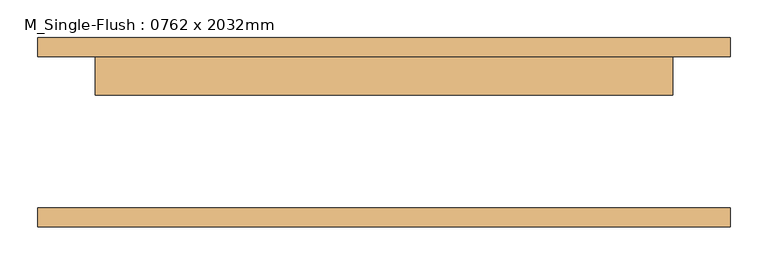
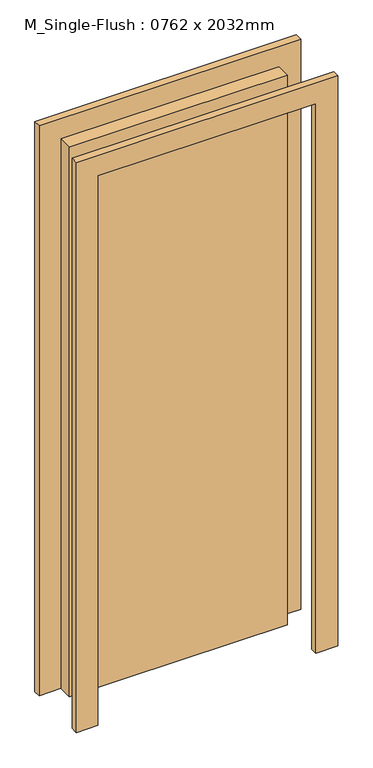
"""IFC4 building model written with IfcOpenShell, lengths in millimetres: door geometry, M_Single-Flush : 0762 x 2032mm."""

from ifc_helpers import new_model, si_unit, frame, origin, origin_with_axes, place, context, project, spatial, polyline, outline, extrude, source, transform, mapped, element, save


def m_single_flush_0762_x_2032mm_0c256fab(model_context):
    return source(origin(), model_context, "Body", "SweptSolid", [
        extrude(outline(polyline([(2108.0, -457.0), (0.0, -457.0), (0.0, -381.0), (2032.0, -381.0), (2032.0, 381.0), (0.0, 381.0), (0.0, 457.0), (2108.0, 457.0), (2108.0, -457.0)])), frame((0.0, 100.0, 0.0), z_axis=(0.0, 1.0, 0.0), x_axis=(0.0, 0.0, 1.0)), (0.0, 0.0, 1.0), 25.0),
        extrude(outline(polyline([(2108.0, 457.0), (2108.0, -457.0), (0.0, -457.0), (0.0, -381.0), (2032.0, -381.0), (2032.0, 381.0), (0.0, 381.0), (0.0, 457.0), (2108.0, 457.0)])), frame((0.0, -125.0, 0.0), z_axis=(0.0, 1.0, 0.0), x_axis=(0.0, 0.0, 1.0)), (0.0, 0.0, 1.0), 25.0),
        extrude(outline(polyline([(381.0, 49.0), (-381.0, 49.0), (-381.0, 100.0), (381.0, 100.0), (381.0, 49.0)])), origin_with_axes(), (0.0, 0.0, 1.0), 2032.0),
    ])


if __name__ == "__main__":
    model = new_model("IFC4")
    model_context = context("Model", 3, world=origin())
    ifc_project = project(units=[si_unit("LENGTHUNIT", "METRE", prefix="MILLI")], contexts=[model_context])
    site = spatial("IfcSite", under=ifc_project)
    building = spatial("IfcBuilding", under=site)
    placement = place(None, origin())
    m_single_flush_0762_x_2032mm_shape = m_single_flush_0762_x_2032mm_0c256fab(model_context)
    element("IfcDoor", 1, ObjectType="M_Single-Flush : 0762 x 2032mm", at=placement, inside=building, context=model_context, shape_type="MappedRepresentation", body=[
        mapped(m_single_flush_0762_x_2032mm_shape, transform((0.0, 0.0, 0.0), x_axis=(1.0, 0.0, 0.0), y_axis=(0.0, 1.0, 0.0), z_axis=(0.0, 0.0, 1.0))),
    ])
    save(model, "model.ifc")

# Revit data of these elements
# Type "M_Single-Flush : 0762 x 2032mm"
#   Type Mark = "19"
#   Thickness = 0' - 2.00787"
#   Height = 6' - 8"
#   Trim Projection Ext = 0' - 0.98425"
#   Trim Projection Int = 0' - 0.98425"
#   Trim Width = 0' - 2.99213"
#   Width = 2' - 6"
#   Door Material = Door - Panel
#   Frame Material = Door - Frame
#   Function = (empty or 0)
#   Wall Closure = (empty or 0)
# Element 1 (IfcDoor, "M_Single-Flush : 0762 x 2032mm")
#   Materials on its faces: "Door - Frame", "Door - Panel"
# Materials
#   "Door - Panel": class "Wood", colour RGB 114 82 51, transparency 0
#   "Door - Frame": colour RGB 153 76 43, transparency 0
